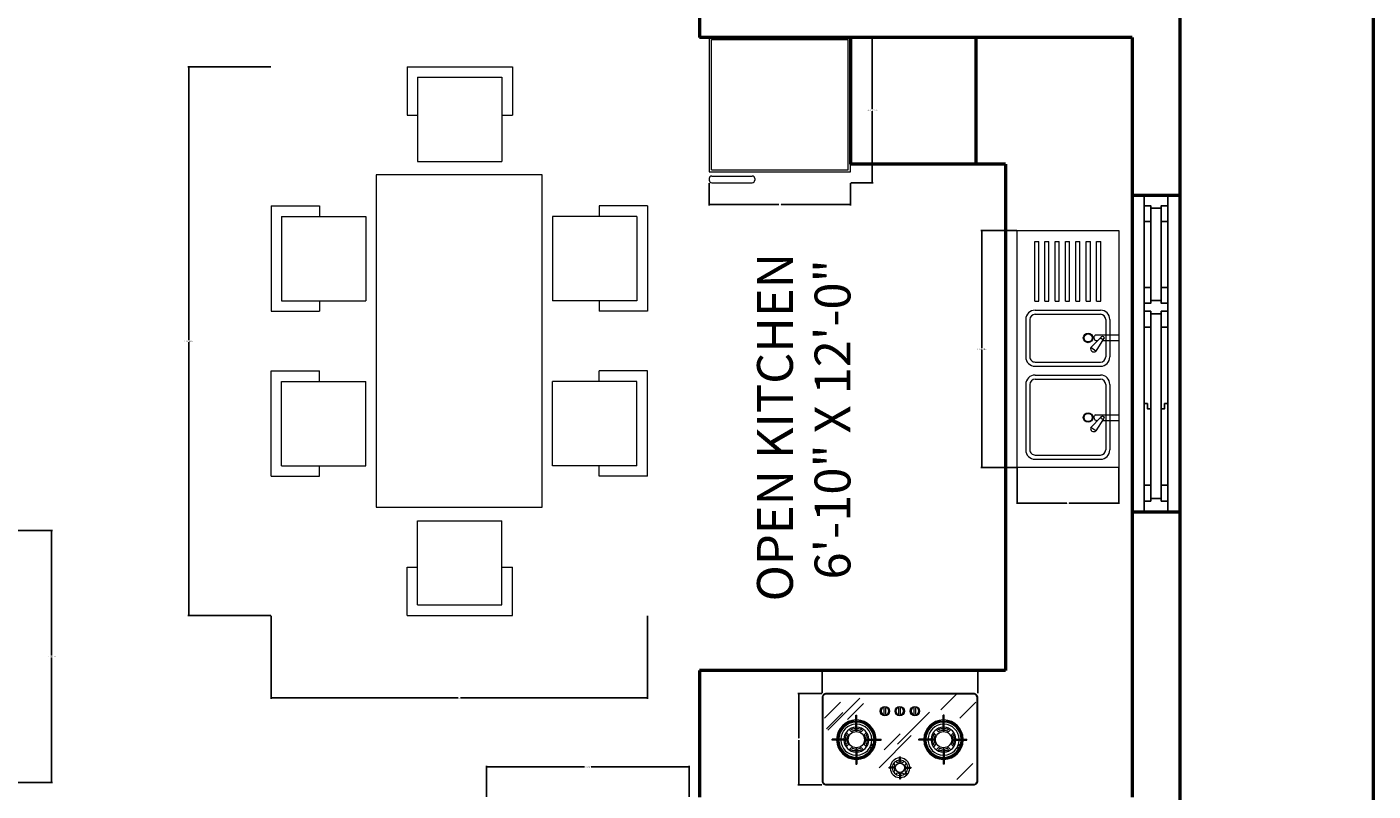
# Model space of a CAD drawing. Units: inches. Extents: x 64 to 1167, y 117 to 939.
# Tile 5 of 56: x 258 to 513, y 438 to 583. Entities that reach past the tile are written whole.
import ezdxf

# ---------------------------------------------------------------- set-up
doc = ezdxf.new("R2010")
doc.units = ezdxf.units.IN
doc.header["$MEASUREMENT"] = 0
for name, color, linetype, lineweight in [('A-ANNO-DIMS', 2, 'Continuous', 18), ('A-ANNO-TEXT', 7, 'Continuous', 25), ('A-ANNO-TTLB', 7, 'Continuous', 50), ('A-FLOR-FIXT', 8, 'Continuous', 18), ('A-FURN', 8, 'Continuous', 18), ('A-GLAZ', 4, 'Continuous', 25), ('A-WALL', 7, 'Continuous', 50)]:
    doc.layers.add(name, color=color, linetype=linetype, lineweight=lineweight)
doc.styles.get("Standard").update_dxf_attribs({"font": 'arial.ttf'})
doc.dimstyles.get("Standard").update_dxf_attribs({"dimtxt": 0.18, "dimasz": 0.18, "dimexe": 0.18, "dimexo": 0.0625, "dimgap": 0.09, "dimtad": 0, "dimtih": 1, "dimtoh": 1, "dimdec": 4, "dimzin": 0, "dimdsep": 46, "dimtxsty": 'Standard', "dimcen": 0.09, "dimadec": 0, "dimazin": 0, "dimtfac": 1, "dimtdec": 4, "dimtofl": 0, "dimtmove": 0, "dimatfit": 3, "dimfxl": 1, "dimtolj": 1, "dimtzin": 0, "dimarcsym": 0})

# ---------------------------------------------------------------- blocks, each defined once
blk = doc.blocks.new('A$C6CB038CA')
for p, q in [((0, 0), (0, 19.23)), ((0, 19.23), (44.91, 19.23)), ((19.79, 14.86), (19.79, 19.23)), ((20.86, 16.25), (20.86, 19.23)), ((34.91, 14.86), (34.91, 19.23)), ((35.98, 16.25), (35.98, 19.23)), ((44.91, 19.23), (44.91, 0)), ((2.05, 15.04), (2.05, 15.83)), ((13.36, 15.83), (2.05, 15.83)), ((13.36, 15.04), (13.36, 15.83)), ((15.09, 3.38), (15.09, 15.78)), ((15.88, 3.38), (15.88, 15.78)), ((16.86, 17.55), (23.95, 17.55)), ((16.86, 16.76), (23.95, 16.76)), ((22.19, 13.93), (20.27, 15.84)), ((20.55, 16.35), (22.84, 14.9)), ((24.94, 3.38), (24.94, 15.78)), ((25.72, 3.38), (25.72, 15.78)), ((27.39, 3.38), (27.39, 15.78)), ((28.18, 3.38), (28.18, 15.78)), ((29.16, 17.55), (41.57, 17.55)), ((29.16, 16.76), (41.57, 16.76)), ((37.31, 13.93), (35.39, 15.84)), ((35.67, 16.35), (37.97, 14.9)), ((42.55, 3.38), (42.55, 15.78)), ((43.34, 3.38), (43.34, 15.78)), ((13.36, 15.04), (2.05, 15.04)), ((2.05, 13.08), (2.05, 13.86)), ((13.36, 13.86), (2.05, 13.86)), ((13.36, 13.08), (2.05, 13.08)), ((13.36, 13.08), (13.36, 13.86)), ((20.86, 14.87), (20.86, 15.26)), ((22.84, 14.9), (22.19, 13.93)), ((35.98, 14.87), (35.98, 15.26)), ((37.97, 14.9), (37.31, 13.93)), ((2.05, 11.11), (2.05, 11.89)), ((13.36, 11.89), (2.05, 11.89)), ((13.36, 11.11), (2.05, 11.11)), ((13.36, 11.11), (13.36, 11.89)), ((2.05, 9.14), (2.05, 9.93)), ((13.36, 9.93), (2.05, 9.93)), ((13.36, 9.14), (2.05, 9.14)), ((2.05, 7.17), (2.05, 7.96)), ((13.36, 7.96), (2.05, 7.96)), ((13.36, 9.14), (13.36, 9.93)), ((13.36, 7.17), (13.36, 7.96)), ((13.36, 7.17), (2.05, 7.17)), ((2.05, 5.2), (2.05, 5.99)), ((13.36, 5.99), (2.05, 5.99)), ((13.36, 5.2), (2.05, 5.2)), ((13.36, 5.2), (13.36, 5.99)), ((2.05, 3.34), (2.05, 4.12)), ((13.36, 4.12), (2.05, 4.12)), ((13.36, 3.34), (2.05, 3.34)), ((13.36, 3.34), (13.36, 4.12)), ((44.91, 0), (0, 0)), ((16.86, 2.39), (23.95, 2.39)), ((16.86, 1.61), (23.95, 1.61)), ((29.16, 2.39), (41.57, 2.39)), ((29.16, 1.61), (41.57, 1.61))]:
    blk.add_line(p, q)
for centre, radius in [((20.33, 16.16), 0.307), ((35.45, 16.16), 0.307), ((20.35, 13.43), 0.909), ((20.35, 13.44), 0.768), ((35.44, 13.43), 0.909), ((35.44, 13.44), 0.768)]:
    blk.add_circle(centre, radius)
for centre, radius, start, end in [((16.86, 15.78), 1.77, 90, 180), ((16.86, 15.78), 0.984, 90, 180), ((23.95, 15.78), 1.77, 0, 90), ((23.95, 15.78), 0.984, 0, 90), ((29.16, 15.78), 1.77, 90, 180), ((29.16, 15.78), 0.984, 90, 180), ((41.57, 15.78), 1.77, 0, 90), ((41.57, 15.78), 0.984, 0, 90), ((20.32, 15.11), 0.586, 205.1043, 335.2171), ((22.39, 14.51), 0.611, 251.2024, 39.3215), ((35.44, 15.11), 0.586, 205.1043, 335.2171), ((37.51, 14.51), 0.611, 251.2024, 39.3215), ((16.86, 3.38), 1.77, 180, 270), ((16.86, 3.38), 0.984, 180, 270), ((23.95, 3.38), 0.984, 270, 0), ((23.95, 3.38), 1.77, 270, 0), ((29.16, 3.38), 1.77, 180, 270), ((29.16, 3.38), 0.984, 180, 270), ((41.57, 3.38), 0.984, 270, 0), ((41.57, 3.38), 1.77, 270, 0)]:
    blk.add_arc(centre, radius, start, end)
blk = doc.blocks.new('A$C038F079D')
for p, q in [((0.94, 13.26), (3.99, 16.31)), ((14.86, 16.17), (14.67, 16.17)), ((12.63, 7.98), (18.73, 14.07)), ((16.82, 14.17), (16.82, 13.97)), ((23.13, 13.38), (22.93, 13.38)), ((14.86, 12.03), (14.67, 12.03)), ((14.73, 7.63), (17.78, 10.68)), ((2.09, 8.85), (2.09, 8.65)), ((9.14, 3.52), (15.23, 9.61)), ((11.18, 8.85), (11.18, 8.65)), ((18.35, 8.85), (18.35, 8.65)), ((27.63, 8.85), (27.63, 8.65)), ((5.13, 6.82), (5.56, 7.25)), ((5.41, 6.65), (5.61, 6.86)), ((22.35, 0.88), (28.44, 6.97)), ((25.61, 3.63), (28.66, 6.68)), ((0.4, 1.61), (3.44, 4.66)), ((3.97, 0.06), (7.02, 3.11)), ((21.65, 1.88), (24.69, 4.93)), ((23.13, 4.08), (22.93, 4.08)), ((26.04, 1.65), (29.08, 4.7))]:
    blk.add_line(p, q)
at = {"ltscale": 0.18}
for p, q in [((14.67, 15.14), (14.67, 16.17)), ((14.86, 15.14), (14.86, 16.17)), ((6.4, 13.38), (6.6, 13.38)), ((6.4, 10.52), (6.4, 13.38)), ((6.6, 10.52), (6.6, 13.38)), ((12.69, 13.97), (12.69, 14.17)), ((13.69, 14.17), (12.69, 14.17)), ((13.69, 13.97), (12.69, 13.97)), ((13.81, 14.57), (13.52, 14.86)), ((13.52, 13.27), (13.81, 13.56)), ((14.26, 15.02), (13.97, 15.31)), ((13.97, 12.83), (14.26, 13.12)), ((14.67, 12.99), (14.67, 12.03)), ((14.86, 12.99), (14.86, 12.03)), ((15.27, 15.02), (15.56, 15.31)), ((15.56, 12.83), (15.27, 13.12)), ((15.72, 14.57), (16, 14.86)), ((16, 13.27), (15.72, 13.56)), ((15.84, 14.17), (16.82, 14.17)), ((15.84, 13.97), (16.82, 13.97)), ((22.93, 10.52), (22.93, 13.38)), ((23.13, 10.52), (23.13, 13.38)), ((5.13, 10.67), (5.56, 10.25)), ((5.41, 10.84), (5.61, 10.64)), ((7.39, 10.64), (7.59, 10.84)), ((7.44, 10.25), (7.87, 10.67)), ((22.09, 10.25), (21.66, 10.67)), ((22.14, 10.64), (21.94, 10.84)), ((24.12, 10.84), (23.92, 10.64)), ((24.4, 10.67), (23.97, 10.25)), ((4.93, 8.85), (2.09, 8.85)), ((4.93, 8.65), (2.09, 8.65)), ((4.4, 9.84), (4.61, 9.64)), ((4.4, 7.66), (4.61, 7.86)), ((4.57, 10.12), (5, 9.69)), ((4.57, 7.38), (5, 7.81)), ((8, 9.69), (8.42, 10.12)), ((8, 7.81), (8.42, 7.38)), ((8.27, 8.85), (11.18, 8.85)), ((8.27, 8.65), (11.18, 8.65)), ((8.39, 9.64), (8.59, 9.84)), ((8.39, 7.86), (8.59, 7.66)), ((21.26, 8.85), (18.35, 8.85)), ((21.26, 8.65), (18.35, 8.65)), ((21.14, 9.64), (20.93, 9.84)), ((21.14, 7.86), (20.93, 7.66)), ((21.53, 9.69), (21.1, 10.12)), ((21.53, 7.81), (21.1, 7.38)), ((24.95, 10.12), (24.53, 9.69)), ((24.95, 7.38), (24.53, 7.81)), ((24.8, 8.85), (27.63, 8.85)), ((24.8, 8.65), (27.63, 8.65)), ((25.12, 9.84), (24.92, 9.64)), ((25.12, 7.66), (24.92, 7.86)), ((6.4, 6.98), (6.4, 4.08)), ((6.6, 6.98), (6.6, 4.08)), ((7.39, 6.86), (7.59, 6.65)), ((7.44, 7.25), (7.87, 6.82)), ((22.09, 7.25), (21.66, 6.82)), ((22.14, 6.86), (21.94, 6.65)), ((22.93, 6.98), (22.93, 4.08)), ((23.13, 6.98), (23.13, 4.08)), ((24.12, 6.65), (23.92, 6.86)), ((24.4, 6.82), (23.97, 7.25)), ((6.4, 4.08), (6.6, 4.08)), ((11.76, 3.93), (11.76, 2.72)), ((12.07, 3.93), (12.07, 2.72)), ((14.64, 3.93), (14.64, 2.72)), ((14.96, 3.93), (14.96, 2.72)), ((17.46, 3.93), (17.46, 2.72)), ((17.77, 3.93), (17.77, 2.72))]:
    blk.add_line(p, q, dxfattribs=at)
for points in [[(0.79, 0), (28.74, 0, 0.414214), (29.53, 0.79), (29.53, 16.54, 0.414214), (28.74, 17.32), (0.79, 17.32, 0.414214), (0, 16.54), (0, 0.79, 0.414214)], [(0.79, 0.12), (28.74, 0.12, 0.414214), (29.41, 0.79), (29.41, 16.54, 0.414214), (28.74, 17.2), (0.79, 17.2, 0.414214), (0.12, 16.54), (0.12, 0.79, 0.414214)]]:
    blk.add_lwpolyline(points, format="xyb", close=True)
for centre in [(13.62, 15.21), (3.73, 10.29), (20.26, 10.27), (3.51, 9.78), (20.04, 9.75)]:
    blk.add_circle(centre, 0.147)
for centre, radius in [((14.76, 14.07), 0.881), ((6.5, 8.75), 1.54), ((23.03, 8.75), 1.54), ((11.92, 3.32), 0.886), ((11.92, 3.32), 0.846), ((14.8, 3.32), 0.886), ((14.8, 3.32), 0.846), ((17.61, 3.32), 0.886), ((17.61, 3.32), 0.846)]:
    blk.add_circle(centre, radius, dxfattribs=at)
for centre, radius, start, end in [((14.76, 14.07), 1.86, 93.0255, 176.9745), ((14.76, 14.07), 1.47, 93.8363, 176.1637), ((14.76, 14.07), 1.86, 3.0255, 86.9745), ((14.76, 14.07), 1.47, 3.8363, 86.1637), ((14.76, 14.07), 1.86, 183.0255, 266.9745), ((14.76, 14.07), 1.47, 183.8363, 266.1637), ((14.76, 14.07), 1.08, 151.9979, 174.8384), ((13.66, 14.07), 0.103, 287.6318, 72.3682), ((14.76, 14.07), 1.08, 185.1616, 208.0021), ((14.76, 14.07), 1.08, 95.203, 118.0021), ((14.76, 14.07), 1.08, 241.9979, 264.7569), ((14.76, 15.16), 0.0994, 187.9505, 352.0495), ((14.76, 12.99), 0.0985, 358.3317, 181.6683), ((14.76, 14.07), 1.08, 61.9979, 84.797), ((14.76, 14.07), 1.86, 273.0255, 356.9745), ((14.76, 14.07), 1.47, 273.8363, 356.1637), ((14.76, 14.07), 1.08, 275.2431, 298.0021), ((14.76, 14.07), 1.08, 5.206, 28.0021), ((14.76, 14.07), 1.08, 331.9979, 354.794), ((15.85, 14.07), 0.0992, 97.2236, 262.7764), ((6.5, 8.75), 3.74, 91.5918, 178.4082), ((6.5, 8.75), 3.54, 91.5918, 178.4082), ((6.5, 8.75), 3.35, 91.6854, 178.3146), ((6.5, 8.75), 2.95, 91.9102, 178.0898), ((6.5, 8.75), 2.36, 92.388, 177.612), ((6.5, 8.75), 1.77, 93.1847, 122.1604), ((6.5, 8.75), 2.09, 92.7036, 115.1461), ((6.5, 10.53), 0.0991, 186.7354, 353.2646), ((6.5, 8.75), 3.74, 1.5918, 88.4082), ((6.5, 8.75), 3.54, 1.5918, 88.4082), ((6.5, 8.75), 3.35, 1.6854, 88.3146), ((6.5, 8.75), 2.95, 1.9102, 88.0898), ((6.5, 8.75), 2.36, 2.388, 87.612), ((6.5, 8.75), 2.09, 64.8539, 87.2964), ((6.5, 8.75), 1.77, 57.8396, 86.8153), ((23.03, 8.75), 3.74, 91.5918, 178.4082), ((23.03, 8.75), 3.54, 91.5918, 178.4082), ((23.03, 8.75), 3.35, 91.6854, 178.3146), ((23.03, 8.75), 2.95, 91.9102, 178.0898), ((23.03, 8.75), 2.36, 92.388, 177.612), ((23.03, 8.75), 1.77, 93.1847, 122.1604), ((23.03, 8.75), 2.09, 92.7036, 115.1461), ((23.03, 10.52), 0.0987, 183.9579, 356.0421), ((23.03, 8.75), 3.74, 1.5918, 88.4082), ((23.03, 8.75), 3.54, 1.5918, 88.4082), ((23.03, 8.75), 3.35, 1.6854, 88.3146), ((23.03, 8.75), 2.95, 1.9102, 88.0898), ((23.03, 8.75), 2.36, 2.388, 87.612), ((23.03, 8.75), 2.09, 64.8539, 87.2964), ((23.03, 8.75), 1.77, 57.8396, 86.8153), ((6.5, 8.75), 3.74, 181.5918, 268.4082), ((6.5, 8.75), 3.54, 181.5918, 268.4082), ((6.5, 8.75), 3.35, 181.6854, 268.3146), ((6.5, 8.75), 2.95, 181.9102, 268.0898), ((6.5, 8.75), 2.36, 182.388, 267.612), ((6.5, 8.75), 2.09, 154.8539, 177.2964), ((6.5, 8.75), 2.09, 182.7036, 205.1461), ((6.5, 8.75), 1.77, 147.8396, 176.8153), ((4.7, 8.75), 0.104, 288.751, 71.249), ((6.5, 8.75), 1.77, 183.1847, 212.1604), ((6.5, 8.75), 2.95, 271.9102, 358.0898), ((6.5, 8.75), 2.36, 272.388, 357.612), ((6.5, 8.75), 3.35, 271.6854, 358.3146), ((6.5, 8.75), 3.54, 271.5918, 358.4082), ((6.5, 8.75), 3.74, 271.5918, 358.4082), ((6.5, 8.75), 1.77, 3.1847, 32.1604), ((6.5, 8.75), 1.77, 327.8396, 356.8153), ((8.3, 8.75), 0.105, 110.5507, 249.4493), ((6.5, 8.75), 2.09, 2.7036, 25.1461), ((6.5, 8.75), 2.09, 334.8539, 357.2964), ((23.03, 8.75), 3.74, 181.5918, 268.4082), ((23.03, 8.75), 3.54, 181.5918, 268.4082), ((23.03, 8.75), 3.35, 181.6854, 268.3146), ((23.03, 8.75), 2.95, 181.9102, 268.0898), ((23.03, 8.75), 2.36, 182.388, 267.612), ((23.03, 8.75), 2.09, 154.8539, 177.2964), ((23.03, 8.75), 2.09, 182.7036, 205.1461), ((23.03, 8.75), 1.77, 147.8396, 176.8153), ((21.23, 8.75), 0.104, 288.412, 71.588), ((23.03, 8.75), 1.77, 183.1847, 212.1604), ((23.03, 8.75), 3.54, 271.5918, 358.4082), ((23.03, 8.75), 3.35, 271.6854, 358.3146), ((23.03, 8.75), 2.95, 271.9102, 358.0898), ((23.03, 8.75), 2.36, 272.388, 357.612), ((23.03, 8.75), 3.74, 271.5918, 358.4082), ((23.03, 8.75), 1.77, 3.1847, 32.1604), ((23.03, 8.75), 1.77, 327.8396, 356.8153), ((24.82, 8.75), 0.102, 104.2945, 255.7055), ((23.03, 8.75), 2.09, 2.7036, 25.1461), ((23.03, 8.75), 2.09, 334.8539, 357.2964), ((6.5, 8.75), 1.77, 237.8396, 266.8153), ((6.5, 8.75), 2.09, 244.8539, 267.2964), ((6.5, 8.75), 1.77, 273.1847, 302.1604), ((6.5, 8.75), 2.09, 272.7036, 295.1461), ((23.03, 8.75), 1.77, 237.8396, 266.8153), ((23.03, 8.75), 2.09, 244.8539, 267.2964), ((23.03, 6.95), 0.103, 17.9418, 162.0582), ((23.03, 8.75), 1.77, 273.1847, 302.1604), ((23.03, 8.75), 2.09, 272.7036, 295.1461), ((11.92, 3.32), 0.728, 111.3237, 248.6763), ((11.68, 3.93), 0.0787, 0, 111.3237), ((11.68, 2.72), 0.0787, 248.6763, 0), ((12.15, 3.93), 0.0787, 68.6763, 180), ((12.15, 2.72), 0.0787, 180, 291.3237), ((11.92, 3.32), 0.728, 291.3237, 68.6763), ((14.8, 3.32), 0.728, 111.3237, 248.6763), ((14.57, 3.93), 0.0787, 0, 111.3237), ((14.57, 2.72), 0.0787, 248.6763, 0), ((15.04, 3.93), 0.0787, 68.6763, 180), ((15.04, 2.72), 0.0787, 180, 291.3237), ((14.8, 3.32), 0.728, 291.3237, 68.6763), ((17.61, 3.32), 0.728, 111.3237, 248.6763), ((17.38, 3.93), 0.0787, 0, 111.3237), ((17.38, 2.72), 0.0787, 248.6763, 0), ((17.85, 3.93), 0.0787, 68.6763, 180), ((17.85, 2.72), 0.0787, 180, 291.3237), ((17.61, 3.32), 0.728, 291.3237, 68.6763)]:
    blk.add_arc(centre, radius, start, end, dxfattribs=at)
blk.add_arc((6.5, 6.94), 0.106, 21.7885, 158.2115)
blk = doc.blocks.new('A$C097D0B75')
for p, q in [((0, 27.53), (0, 2.04)), ((0, 27.53), (26.77, 27.53)), ((0.43, 2.43), (0.43, 27.14)), ((0.43, 27.14), (26.35, 27.14)), ((26.35, 2.43), (26.35, 27.14)), ((26.77, 2.04), (26.77, 27.53)), ((0, 2.04), (26.77, 2.04)), ((0, 0.78), (0, 0.49)), ((0.43, 2.43), (26.35, 2.43)), ((0.49, 1.27), (8.14, 1.27)), ((0.49, 0), (8.14, 0)), ((8.64, 0.78), (8.64, 0.49))]:
    blk.add_line(p, q)
for centre, start, end in [((0.49, 0.78), 90, 180), ((0.49, 0.49), 180, 270), ((8.14, 0.78), 0, 90), ((8.14, 0.49), 270, 0)]:
    blk.add_arc(centre, 0.494, start, end)
blk = doc.blocks.new('A$C30E17696')
for p, q in [((0.02639, 0.07131), (0.04634, 0.07131)), ((0.02639, 0.07131), (0.02639, 0.06215)), ((0.02838, 0.06931), (0.02838, 0.05336)), ((0.02838, 0.06931), (0.04434, 0.06931)), ((0.04434, 0.06931), (0.04434, 0.05336)), ((0.04634, 0.07131), (0.04634, 0.06215)), ((0.0776, 0.07131), (0.05766, 0.07131)), ((0.05766, 0.07131), (0.05766, 0.06215)), ((0.05965, 0.06931), (0.05965, 0.05336)), ((0.07561, 0.06931), (0.05965, 0.06931)), ((0.07561, 0.06931), (0.07561, 0.05336)), ((0.0776, 0.07131), (0.0776, 0.06215)), ((0.02639, 0.06215), (0.02838, 0.06215)), ((0.04434, 0.06215), (0.04634, 0.06215)), ((0.05965, 0.06215), (0.05766, 0.06215)), ((0.0776, 0.06215), (0.07561, 0.06215)), ((0.0205, 0.0514), (0.0205, 0.01991)), ((0.08349, 0.0514), (0.0205, 0.0514)), ((0.02838, 0.05336), (0.04434, 0.05336)), ((0.07561, 0.05336), (0.05965, 0.05336)), ((0.08349, 0.01991), (0.08349, 0.0514)), ((0, 0.02577), (0, 0.04572)), ((0, 0.04572), (0.00916, 0.04572)), ((0.00199, 0.02776), (0.00199, 0.04372)), ((0.00199, 0.04372), (0.01795, 0.04372)), ((0.00916, 0.04372), (0.00916, 0.04572)), ((0.01795, 0.02776), (0.01795, 0.04372)), ((0.08604, 0.02776), (0.08604, 0.04372)), ((0.102, 0.04372), (0.08604, 0.04372)), ((0.10399, 0.04572), (0.09483, 0.04572)), ((0.09483, 0.04372), (0.09483, 0.04572)), ((0.102, 0.02776), (0.102, 0.04372)), ((0.10399, 0.02577), (0.10399, 0.04572)), ((0, 0.02577), (0.00916, 0.02577)), ((0.00199, 0.02776), (0.01795, 0.02776)), ((0.00916, 0.02577), (0.00916, 0.02776)), ((0.102, 0.02776), (0.08604, 0.02776)), ((0.09483, 0.02577), (0.09483, 0.02776)), ((0.10399, 0.02577), (0.09483, 0.02577)), ((0.0205, 0.01991), (0.08349, 0.01991)), ((0.02838, 0.01795), (0.04434, 0.01795)), ((0.02838, 0.00199), (0.02838, 0.01795)), ((0.04434, 0.00199), (0.04434, 0.01795)), ((0.05965, 0.00199), (0.05965, 0.01795)), ((0.07561, 0.01795), (0.05965, 0.01795)), ((0.07561, 0.00199), (0.07561, 0.01795)), ((0.02639, 0), (0.02639, 0.00916)), ((0.02639, 0.00916), (0.02838, 0.00916)), ((0.04434, 0.00916), (0.04634, 0.00916)), ((0.04634, 0), (0.04634, 0.00916)), ((0.05766, 0), (0.05766, 0.00916)), ((0.05965, 0.00916), (0.05766, 0.00916)), ((0.0776, 0.00916), (0.07561, 0.00916)), ((0.0776, 0), (0.0776, 0.00916)), ((0.02838, 0.00199), (0.04434, 0.00199)), ((0.07561, 0.00199), (0.05965, 0.00199)), ((0.02639, 0), (0.04634, 0)), ((0.0776, 0), (0.05766, 0))]:
    blk.add_line(p, q)
blk = doc.blocks.new("W-5'")
for p, q in [((0, 9), (0, 0)), ((0, 9), (60, 9)), ((60, 9), (60, 0)), ((0, 6.75), (60, 6.75)), ((2, 5.5), (20.5, 5.5)), ((58, 5.5), (22, 5.5)), ((2, 3.5), (20.5, 3.5)), ((58, 3.5), (22, 3.5)), ((0, 2.25), (60, 2.25)), ((0, 0), (60, 0))]:
    blk.add_line(p, q)
for points in [[(0, 2.25), (0, 6.75), (2, 6.75), (2, 5.5), (2.5, 5.5), (2.5, 3.5), (2, 3.5), (2, 2.25), (0, 2.25)], [(5, 6.75), (5, 5.5)], [(17.5, 6.75), (17.5, 5.5)], [(25, 6.75), (25, 5.5)], [(39.5, 6.75), (39.5, 6.125), (40.5, 6.125), (40.5, 5.5)], [(55, 6.75), (55, 5.5)], [(60, 2.25), (60, 6.75), (58, 6.75), (58, 5.5), (57.5, 5.5), (57.5, 3.5), (58, 3.5), (58, 2.25), (60, 2.25)], [(5, 3.5), (5, 2.25)], [(17.5, 3.5), (17.5, 2.25)], [(25, 3.5), (25, 2.25)], [(39.5, 2.25), (39.5, 2.875), (40.5, 2.875), (40.5, 3.5)], [(55, 3.5), (55, 2.25)]]:
    blk.add_lwpolyline(points)
blk.add_lwpolyline([(22, 6.75), (20.5, 6.75), (20.5, 5.5), (20, 5.5), (20, 3.5), (20.5, 3.5), (20.5, 2.25), (22, 2.25), (22, 3.5), (22.5, 3.5), (22.5, 5.5), (22, 5.5)], close=True)
blk = doc.blocks.new('*D58')
at = {"layer": 'A-ANNO-DIMS', "color": 0, "lineweight": -2, "transparency": 16777216}
for p, q in [((255.17, 487.78), (262.45, 487.78)), ((262.27, 487.6), (262.27, 464.08)), ((262.27, 440.19), (262.27, 463.71)), ((255.17, 440.01), (262.45, 440.01))]:
    blk.add_line(p, q, dxfattribs=at)
for points in [[(262.24, 487.6), (262.3, 487.6), (262.27, 487.78)], [(262.24, 440.19), (262.3, 440.19), (262.27, 440.01)]]:
    blk.add_solid(points, dxfattribs=at)
at = {"layer": 'Defpoints', "color": 0, "lineweight": -2, "transparency": 16777216}
for p in [(255.11, 487.78), (255.11, 440.01), (262.27, 440.01)]:
    blk.add_point(p, dxfattribs=at)
at = {"layer": 'A-ANNO-DIMS', "color": 0, "transparency": 16777216, "insert": (262.27, 463.9), "char_height": 0.18, "attachment_point": 5}
blk.add_mtext('\\A1;DOOR 48 TYP.', dxfattribs=at)
blk = doc.blocks.new('*D62')
at = {"layer": 'A-ANNO-DIMS', "color": 0, "lineweight": -2, "transparency": 16777216}
for p, q in [((344.69, 437.26), (344.69, 443.15)), ((344.87, 442.97), (363.29, 442.97)), ((382.96, 442.97), (364.54, 442.97)), ((383.14, 437.26), (383.14, 443.15))]:
    blk.add_line(p, q, dxfattribs=at)
for points in [[(344.87, 443), (344.87, 442.94), (344.69, 442.97)], [(382.96, 443), (382.96, 442.94), (383.14, 442.97)]]:
    blk.add_solid(points, dxfattribs=at)
at = {"layer": 'Defpoints', "color": 0, "lineweight": -2, "transparency": 16777216}
for p in [(344.69, 442.97), (344.69, 437.2), (383.14, 437.2)]:
    blk.add_point(p, dxfattribs=at)
at = {"layer": 'A-ANNO-DIMS', "color": 0, "transparency": 16777216, "insert": (363.91, 442.97), "char_height": 0.18, "attachment_point": 5}
blk.add_mtext('\\A1;DOOR 38', dxfattribs=at)
blk = doc.blocks.new('*D86')
at = {"layer": 'A-ANNO-DIMS', "color": 0, "lineweight": -2, "transparency": 16777216}
for p, q in [((303.84, 575.65), (288.13, 575.65)), ((288.31, 575.47), (288.31, 523.84)), ((288.31, 471.84), (288.31, 523.47)), ((303.84, 471.66), (288.13, 471.66))]:
    blk.add_line(p, q, dxfattribs=at)
for points in [[(288.28, 575.47), (288.34, 575.47), (288.31, 575.65)], [(288.28, 471.84), (288.34, 471.84), (288.31, 471.66)]]:
    blk.add_solid(points, dxfattribs=at)
at = {"layer": 'Defpoints', "color": 0, "lineweight": -2, "transparency": 16777216}
for p in [(303.9, 575.65), (288.31, 471.66), (303.9, 471.66)]:
    blk.add_point(p, dxfattribs=at)
at = {"layer": 'A-ANNO-DIMS', "color": 0, "transparency": 16777216, "insert": (288.31, 523.65), "char_height": 0.18, "attachment_point": 5}
blk.add_mtext('\\A1;DINING SET 104', dxfattribs=at)
blk = doc.blocks.new('*D87')
at = {"layer": 'A-ANNO-DIMS', "color": 0, "lineweight": -2, "transparency": 16777216}
for p, q in [((303.9, 471.6), (303.9, 455.88)), ((375.21, 471.6), (375.21, 455.88)), ((304.08, 456.06), (339.36, 456.06)), ((375.03, 456.06), (339.76, 456.06))]:
    blk.add_line(p, q, dxfattribs=at)
for points in [[(304.08, 456.09), (304.08, 456.03), (303.9, 456.06)], [(375.03, 456.09), (375.03, 456.03), (375.21, 456.06)]]:
    blk.add_solid(points, dxfattribs=at)
at = {"layer": 'Defpoints', "color": 0, "lineweight": -2, "transparency": 16777216}
for p in [(303.9, 471.66), (375.21, 471.66), (375.21, 456.06)]:
    blk.add_point(p, dxfattribs=at)
at = {"layer": 'A-ANNO-DIMS', "color": 0, "transparency": 16777216, "insert": (339.56, 456.06), "char_height": 0.18, "attachment_point": 5}
blk.add_mtext('\\A1;71', dxfattribs=at)
blk = doc.blocks.new('*D88')
at = {"layer": 'A-ANNO-DIMS', "color": 0, "lineweight": -2, "transparency": 16777216}
for p, q in [((445.25, 544.61), (438.4, 544.61)), ((438.58, 544.43), (438.58, 522.33)), ((438.58, 499.88), (438.58, 521.97)), ((445.25, 499.7), (438.4, 499.7))]:
    blk.add_line(p, q, dxfattribs=at)
for points in [[(438.55, 544.43), (438.61, 544.43), (438.58, 544.61)], [(438.55, 499.88), (438.61, 499.88), (438.58, 499.7)]]:
    blk.add_solid(points, dxfattribs=at)
at = {"layer": 'Defpoints', "color": 0, "lineweight": -2, "transparency": 16777216}
for p in [(445.32, 544.61), (438.58, 499.7), (445.32, 499.7)]:
    blk.add_point(p, dxfattribs=at)
at = {"layer": 'A-ANNO-DIMS', "color": 0, "transparency": 16777216, "insert": (438.58, 522.15), "char_height": 0.18, "attachment_point": 5}
blk.add_mtext('\\A1;KITCHEN SINK 45', dxfattribs=at)
blk = doc.blocks.new('*D89')
at = {"layer": 'A-ANNO-DIMS', "color": 0, "lineweight": -2, "transparency": 16777216}
for p, q in [((445.32, 499.63), (445.32, 492.78)), ((464.55, 499.63), (464.55, 492.78)), ((445.5, 492.96), (454.72, 492.96)), ((464.37, 492.96), (455.14, 492.96))]:
    blk.add_line(p, q, dxfattribs=at)
for points in [[(445.5, 492.99), (445.5, 492.93), (445.32, 492.96)], [(464.37, 492.99), (464.37, 492.93), (464.55, 492.96)]]:
    blk.add_solid(points, dxfattribs=at)
at = {"layer": 'Defpoints', "color": 0, "lineweight": -2, "transparency": 16777216}
for p in [(445.32, 499.7), (464.55, 499.7), (464.55, 492.96)]:
    blk.add_point(p, dxfattribs=at)
at = {"layer": 'A-ANNO-DIMS', "color": 0, "transparency": 16777216, "insert": (454.93, 492.96), "char_height": 0.18, "attachment_point": 5}
blk.add_mtext('\\A1;19', dxfattribs=at)
blk = doc.blocks.new('*D90')
at = {"layer": 'A-ANNO-DIMS', "color": 0, "lineweight": -2, "transparency": 16777216}
for p, q in [((408.32, 456.92), (408.32, 461.47)), ((408.5, 461.29), (422.56, 461.29)), ((437.67, 461.29), (423.61, 461.29)), ((437.85, 456.92), (437.85, 461.47))]:
    blk.add_line(p, q, dxfattribs=at)
for points in [[(408.5, 461.32), (408.5, 461.26), (408.32, 461.29)], [(437.67, 461.32), (437.67, 461.26), (437.85, 461.29)]]:
    blk.add_solid(points, dxfattribs=at)
at = {"layer": 'Defpoints', "color": 0, "lineweight": -2, "transparency": 16777216}
for p in [(408.32, 461.29), (408.32, 456.86), (437.85, 456.86)]:
    blk.add_point(p, dxfattribs=at)
at = {"layer": 'A-ANNO-DIMS', "color": 0, "transparency": 16777216, "insert": (423.09, 461.29), "char_height": 0.18, "attachment_point": 5}
blk.add_mtext('\\A1;HOB 30', dxfattribs=at)
blk = doc.blocks.new('*D91')
at = {"layer": 'A-ANNO-DIMS', "color": 0, "lineweight": -2, "transparency": 16777216}
for p, q in [((408.26, 456.86), (403.71, 456.86)), ((403.89, 456.68), (403.89, 448.38)), ((403.89, 439.72), (403.89, 448.02)), ((408.26, 439.54), (403.71, 439.54))]:
    blk.add_line(p, q, dxfattribs=at)
for points in [[(403.86, 456.68), (403.92, 456.68), (403.89, 456.86)], [(403.86, 439.72), (403.92, 439.72), (403.89, 439.54)]]:
    blk.add_solid(points, dxfattribs=at)
at = {"layer": 'Defpoints', "color": 0, "lineweight": -2, "transparency": 16777216}
for p in [(408.32, 456.86), (403.89, 439.54), (408.32, 439.54)]:
    blk.add_point(p, dxfattribs=at)
at = {"layer": 'A-ANNO-DIMS', "color": 0, "transparency": 16777216, "insert": (403.89, 448.2), "char_height": 0.18, "attachment_point": 5}
blk.add_mtext('\\A1;17', dxfattribs=at)
blk = doc.blocks.new('*D92')
at = {"layer": 'A-ANNO-DIMS', "color": 0, "lineweight": -2, "transparency": 16777216}
for p, q in [((413.78, 581.2), (418.02, 581.2)), ((417.84, 581.02), (417.84, 567.62)), ((417.84, 553.85), (417.84, 567.25)), ((413.78, 553.67), (418.02, 553.67))]:
    blk.add_line(p, q, dxfattribs=at)
for points in [[(417.81, 581.02), (417.87, 581.02), (417.84, 581.2)], [(417.81, 553.85), (417.87, 553.85), (417.84, 553.67)]]:
    blk.add_solid(points, dxfattribs=at)
at = {"layer": 'Defpoints', "color": 0, "lineweight": -2, "transparency": 16777216}
for p in [(413.71, 581.2), (417.84, 581.2), (413.71, 553.67)]:
    blk.add_point(p, dxfattribs=at)
at = {"layer": 'A-ANNO-DIMS', "color": 0, "transparency": 16777216, "insert": (417.84, 567.43), "char_height": 0.18, "attachment_point": 5}
blk.add_mtext('\\A1;REFRIGERATOR 28', dxfattribs=at)
blk = doc.blocks.new('*D93')
at = {"layer": 'A-ANNO-DIMS', "color": 0, "lineweight": -2, "transparency": 16777216}
for p, q in [((386.94, 553.6), (386.94, 549.36)), ((413.71, 553.6), (413.71, 549.36)), ((387.12, 549.54), (400.11, 549.54)), ((413.53, 549.54), (400.55, 549.54))]:
    blk.add_line(p, q, dxfattribs=at)
for points in [[(387.12, 549.57), (387.12, 549.51), (386.94, 549.54)], [(413.53, 549.57), (413.53, 549.51), (413.71, 549.54)]]:
    blk.add_solid(points, dxfattribs=at)
at = {"layer": 'Defpoints', "color": 0, "lineweight": -2, "transparency": 16777216}
for p in [(386.94, 553.67), (413.71, 553.67), (413.71, 549.54)]:
    blk.add_point(p, dxfattribs=at)
at = {"layer": 'A-ANNO-DIMS', "color": 0, "transparency": 16777216, "insert": (400.33, 549.54), "char_height": 0.18, "attachment_point": 5}
blk.add_mtext('\\A1;27', dxfattribs=at)

msp = doc.modelspace()

# ---------------------------------------------------------------- linework, layer by layer
at = {"layer": 'A-ANNO-TTLB'}
msp.add_lwpolyline([(64.31, 939.22), (512.77, 939.22), (512.77, 116.55), (64.31, 116.55)], close=True, dxfattribs=at)
at = {"layer": 'A-WALL'}
for p, q in [((476.11, 863.2), (476.11, 155.2)), ((385.11, 590.79), (385.11, 581.2)), ((467.11, 581.2), (385.11, 581.2)), ((413.71, 581.2), (413.71, 557.2)), ((437.46, 581.2), (437.46, 557.2)), ((467.11, 581.2), (467.11, 437.2)), ((443.11, 557.2), (413.71, 557.2)), ((443.11, 557.2), (443.11, 461.2)), ((467.11, 551.32), (476.11, 551.32)), ((467.11, 491.32), (476.11, 491.32)), ((443.11, 461.2), (385.11, 461.2)), ((385.11, 461.2), (385.11, 437.2))]:
    msp.add_line(p, q, dxfattribs=at)

# ---------------------------------------------------------------- block references
at = {"layer": 'A-FLOR-FIXT'}
msp.add_blockref('A$C097D0B75', (386.94, 553.67), dxfattribs=at)
for name, p, rotation in [('A$C6CB038CA', (445.32, 544.61), 270), ('A$C038F079D', (437.85, 456.86), 180)]:
    msp.add_blockref(name, p, dxfattribs=dict(at, rotation=rotation))
at = {"layer": 'A-FURN', "xscale": 1000, "yscale": 1000, "zscale": 1000, "rotation": 270}
msp.add_blockref('A$C30E17696', (303.9, 575.65), dxfattribs=at)
at = {"layer": 'A-GLAZ', "rotation": 270}
msp.add_blockref("W-5'", (467.11, 551.32), dxfattribs=at)

# ---------------------------------------------------------------- texts
at = {"layer": 'A-ANNO-TEXT'}
for s, p in [('OPEN KITCHEN', (402.79, 474.32)), ('  6\'-10" X 12\'-0"', (413.7, 474.32))]:
    msp.add_text(s, height=6.7927, rotation=90, dxfattribs=at).set_placement(p)

# ---------------------------------------------------------------- dimensions: what is measured, and where the dimension line sits
at = {"layer": 'A-ANNO-DIMS'}
for base, p1, p2, angle, text, picture, middle in [((417.84, 581.2), (413.71, 553.67), (413.71, 581.2), 90, 'REFRIGERATOR <>', '*D92', (417.84, 567.43)), ((288.31, 471.66), (303.9, 575.65), (303.9, 471.66), 270, 'DINING SET <>', '*D86', (288.31, 523.65)), ((438.58, 499.7), (445.32, 544.61), (445.32, 499.7), 270, 'KITCHEN SINK <>', '*D88', (438.58, 522.15)), ((262.27, 440.01), (255.11, 487.78), (255.11, 440.01), 270, 'DOOR <> TYP.', '*D58', (262.27, 463.9)), ((408.32, 461.29), (437.85, 456.86), (408.32, 456.86), 180, 'HOB <>', '*D90', (423.09, 461.29)), ((344.69, 442.97), (383.14, 437.2), (344.69, 437.2), 180, 'DOOR <>', '*D62', (363.91, 442.97))]:
    dim = msp.add_linear_dim(base=base, p1=p1, p2=p2, angle=angle, text=text, dimstyle='Standard', override={"dimdec": 0, "dimlfac": 1, "dimrnd": 0, "dimzin": 0, "dimdsep": 46, "dimlunit": 2}, dxfattribs=at)
    dim.commit()
    dim.dimension.update_dxf_attribs({"geometry": picture, "text_midpoint": middle})
for base, p1, p2, picture, middle in [((413.71, 549.54), (386.94, 553.67), (413.71, 553.67), '*D93', (400.33, 549.54)), ((464.55, 492.96), (445.32, 499.7), (464.55, 499.7), '*D89', (454.93, 492.96)), ((375.21, 456.06), (303.9, 471.66), (375.21, 471.66), '*D87', (339.56, 456.06))]:
    dim = msp.add_linear_dim(base=base, p1=p1, p2=p2, dimstyle='Standard', override={"dimdec": 0, "dimlfac": 1, "dimrnd": 0, "dimzin": 0, "dimdsep": 46, "dimlunit": 2}, dxfattribs=at)
    dim.commit()
    dim.dimension.update_dxf_attribs({"geometry": picture, "text_midpoint": middle})
dim = msp.add_linear_dim(base=(403.89, 439.54), p1=(408.32, 456.86), p2=(408.32, 439.54), angle=270, dimstyle='Standard', override={"dimdec": 0, "dimlfac": 1, "dimrnd": 0, "dimzin": 0, "dimdsep": 46, "dimlunit": 2}, dxfattribs=at)
dim.commit()
dim.dimension.update_dxf_attribs({"geometry": '*D91', "text_midpoint": (403.89, 448.2)})

doc.saveas('drawing.dxf')
